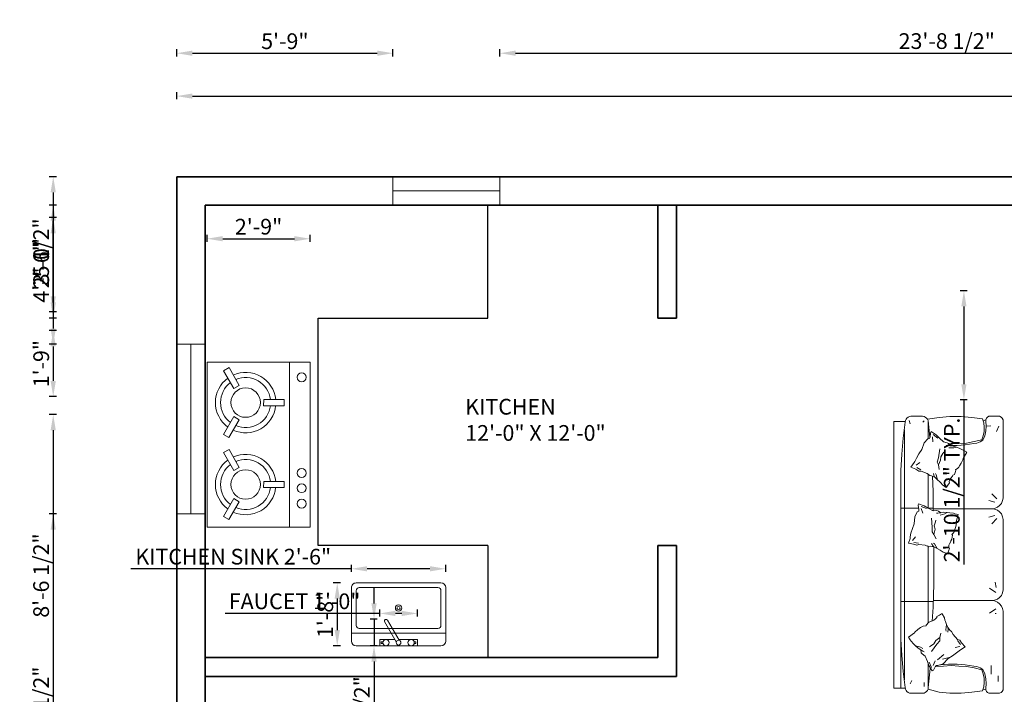
# Model space of a CAD drawing. Units: inches. Extents: x -48 to 817, y -530 to 78.
# Tile 3 of 7: x -48 to 266, y -153 to 62. Entities that reach past the tile are written whole.
import ezdxf

# ---------------------------------------------------------------- set-up
doc = ezdxf.new("R2010")
doc.units = ezdxf.units.IN
for name, color, linetype, lineweight in [('A-ANNO-DIMS', 2, 'Continuous', 18), ('A-AREA-IDEN', 7, 'Continuous', 18), ('A-EQPM', 8, 'Continuous', 18), ('A-FLOR-CASE', 8, 'Continuous', 25), ('A-FLOR-FIXT', 9, 'Continuous', 18), ('A-GLAZ', 4, 'Continuous', 18), ('A-WALL', 7, 'Continuous', 35), ('furn', 8, 'Continuous', 18)]:
    doc.layers.add(name, color=color, linetype=linetype, lineweight=lineweight)
doc.styles.get("Standard").update_dxf_attribs({"font": 'arial.ttf'})
doc.dimstyles.new('ISO-25', dxfattribs={"dimtxt": 5, "dimasz": 5, "dimexe": 1.25, "dimexo": 0.625, "dimtad": 1, "dimlunit": 3, "dimtxsty": 'Standard', "dimcen": 2.5, "dimadec": 0, "dimazin": 0, "dimtfac": 1, "dimtmove": 0, "dimatfit": 3, "dimfxl": 1, "dimfxlon": 1, "dimarcsym": 0})

# ---------------------------------------------------------------- blocks, each defined once
blk = doc.blocks.new('Sink-single - 30 in top')
blk.add_line((-15, -3.999996), (15, -3.999996))
for points in [[(-13.5, 0), (13.5, 0)], [(-15, -18.499996), (-15, -1.5)], [(15, -1.5), (15, -18.499996)], [(-12.5, -5.499996), (12.5, -5.499996)], [(-13.5, -17.499996), (-13.5, -6.499996)], [(13.5, -6.499996), (13.5, -17.499996)], [(12.5, -18.499996), (-12.5, -18.499996)], [(13.5, -19.999996), (-13.5, -19.999996)]]:
    blk.add_lwpolyline(points)
for radius in [1, 0.5]:
    blk.add_circle((0, -11.999996), radius)
for centre, radius, start, end in [((-13.5, -1.5), 1.5, 90, 180), ((13.5, -1.5), 1.5, 0, 90), ((-12.5, -6.499996), 1, 90, 180), ((12.5, -6.499996), 1, 0, 90), ((-13.5, -18.499996), 1.5, 180, 270), ((-12.5, -17.499996), 1, 180, 270), ((12.5, -17.499996), 1, 270, 0), ((13.5, -18.499996), 1.5, 270, 0)]:
    blk.add_arc(centre, radius, start, end)
blk = doc.blocks.new('Faucet - kit sink top')
for p, q in [((-5.5, -0.75), (-5.5, -1.25)), ((-4.94278, -0.75), (-5.5, -0.75)), ((-5.5, -1.25), (-4.94278, -1.25)), ((-0.14775, -1.7441), (3.56698, -8.1782)), ((4.43301, -7.6782), (0.71828, -1.2441)), ((4.94278, -0.75), (5.5, -0.75)), ((5.5, -1.25), (4.94278, -1.25)), ((5.5, -0.75), (5.5, -1.25))]:
    blk.add_line(p, q)
blk.add_lwpolyline([(-0.00587, -2), (-6, -2), (-6, 0), (6, 0), (6, -2), (1.15195, -2)])
for centre, radius in [((-4, -1), 1), ((4, -1), 1), ((0, -1), 0.75)]:
    blk.add_circle(centre, radius)
blk.add_arc((4, -7.9282), 0.5, 210, 30)
blk = doc.blocks.new('sofa-43')
at = {"color": 0, "linetype": 'ByBlock'}
for p, q in [((-0.015, 0.947), (-0.028, 0.939)), ((-0.028, 0.939), (-0.015, 0.947)), ((-0.003, 0.947), (-0.015, 0.947)), ((-0.015, 0.947), (-0.003, 0.947)), ((0.665, 0.947), (-0.003, 0.947)), ((-0.003, 0.947), (0.665, 0.947)), ((0.687, 0.942), (0.665, 0.947)), ((0.687, 0.942), (0.665, 0.947)), ((0.712, 0.932), (0.687, 0.942)), ((0.712, 0.932), (0.687, 0.942)), ((0.827, 0.942), (0.802, 0.932)), ((0.802, 0.932), (0.827, 0.942)), ((0.85, 0.947), (0.827, 0.942)), ((0.827, 0.942), (0.85, 0.947)), ((1.462, 0.947), (0.85, 0.947)), ((0.85, 0.947), (1.462, 0.947)), ((1.487, 0.942), (1.462, 0.947)), ((1.487, 0.942), (1.462, 0.947)), ((1.509, 0.932), (1.487, 0.942)), ((1.509, 0.932), (1.487, 0.942)), ((1.624, 0.942), (1.602, 0.932)), ((1.602, 0.932), (1.624, 0.942)), ((1.647, 0.947), (1.624, 0.942)), ((1.624, 0.942), (1.647, 0.947)), ((2.317, 0.947), (1.647, 0.947)), ((1.647, 0.947), (2.317, 0.947)), ((2.329, 0.947), (2.317, 0.947)), ((2.329, 0.947), (2.317, 0.947)), ((2.342, 0.939), (2.329, 0.947)), ((2.342, 0.939), (2.329, 0.947)), ((-0.038, 0.929), (-0.045, 0.917)), ((-0.045, 0.917), (-0.038, 0.929)), ((-0.045, 0.917), (-0.045, 0.824)), ((-0.045, 0.917), (-0.045, 0.824)), ((-0.028, 0.939), (-0.038, 0.929)), ((-0.038, 0.929), (-0.028, 0.939)), ((0.042, 0.909), (0.087, 0.889)), ((0.672, 0.892), (0.627, 0.849)), ((0.7, 0.874), (0.685, 0.824)), ((0.73, 0.917), (0.712, 0.932)), ((0.73, 0.917), (0.712, 0.932)), ((0.745, 0.897), (0.73, 0.917)), ((0.745, 0.897), (0.73, 0.917)), ((0.755, 0.872), (0.745, 0.897)), ((0.755, 0.872), (0.745, 0.897)), ((0.757, 0.849), (0.755, 0.872)), ((0.757, 0.849), (0.755, 0.872)), ((0.76, 0.872), (0.757, 0.849)), ((0.757, 0.849), (0.76, 0.872)), ((0.77, 0.897), (0.76, 0.872)), ((0.76, 0.872), (0.77, 0.897)), ((0.785, 0.917), (0.77, 0.897)), ((0.77, 0.897), (0.785, 0.917)), ((0.802, 0.932), (0.785, 0.917)), ((0.785, 0.917), (0.802, 0.932)), ((0.815, 0.874), (0.83, 0.824)), ((0.842, 0.892), (0.887, 0.849)), ((1.442, 0.887), (1.394, 0.877)), ((1.484, 0.884), (1.447, 0.829)), ((1.527, 0.917), (1.509, 0.932)), ((1.527, 0.917), (1.509, 0.932)), ((1.542, 0.897), (1.527, 0.917)), ((1.542, 0.897), (1.527, 0.917)), ((1.552, 0.872), (1.542, 0.897)), ((1.552, 0.872), (1.542, 0.897)), ((1.554, 0.849), (1.552, 0.872)), ((1.554, 0.849), (1.552, 0.872)), ((1.557, 0.872), (1.554, 0.849)), ((1.554, 0.849), (1.557, 0.872)), ((1.567, 0.897), (1.557, 0.872)), ((1.557, 0.872), (1.567, 0.897)), ((1.582, 0.917), (1.567, 0.897)), ((1.567, 0.897), (1.582, 0.917)), ((1.602, 0.932), (1.582, 0.917)), ((1.582, 0.917), (1.602, 0.932)), ((1.627, 0.884), (1.664, 0.829)), ((1.667, 0.887), (1.667, 0.877)), ((2.257, 0.904), (2.207, 0.904)), ((2.352, 0.929), (2.342, 0.939)), ((2.352, 0.929), (2.342, 0.939)), ((2.359, 0.917), (2.352, 0.929)), ((2.359, 0.917), (2.352, 0.929)), ((2.359, 0.824), (2.359, 0.917)), ((2.359, 0.917), (2.359, 0.824)), ((-0.045, 0.824), (-0.038, 0.812)), ((-0.045, 0.824), (-0.038, 0.812)), ((-0.038, 0.812), (-0.028, 0.802)), ((-0.038, 0.812), (-0.028, 0.802)), ((-0.023, 0.769), (-0.035, 0.677)), ((-0.023, 0.769), (-0.035, 0.677)), ((-0.028, 0.802), (-0.015, 0.797)), ((-0.028, 0.802), (-0.015, 0.797)), ((0.012, 0.779), (-0.023, 0.769)), ((-0.0064, 0.7737), (-0.023, 0.769)), ((-0.015, 0.797), (-0.0064, 0.7737)), ((-0.015, 0.797), (-0.003, 0.797)), ((-0.0064, 0.7737), (-0.015, 0.797)), ((0.04, 0.799), (-0.003, 0.797)), ((0.05, 0.782), (0.012, 0.779)), ((0.04, 0.799), (0.037, 0.839)), ((0.082, 0.797), (0.04, 0.799)), ((0.087, 0.782), (0.05, 0.782)), ((0.125, 0.787), (0.082, 0.797)), ((0.125, 0.774), (0.087, 0.782)), ((0.162, 0.772), (0.125, 0.787)), ((0.16, 0.762), (0.125, 0.774)), ((0.177, 0.747), (0.162, 0.772)), ((0.757, 0.345), (0.757, 0.849)), ((1.554, 0.345), (1.554, 0.849)), ((2.194, 0.842), (2.119, 0.842)), ((2.137, 0.747), (2.152, 0.772)), ((2.152, 0.772), (2.189, 0.787)), ((2.154, 0.762), (2.189, 0.774)), ((2.189, 0.787), (2.232, 0.797)), ((2.189, 0.774), (2.227, 0.782)), ((2.227, 0.782), (2.264, 0.782)), ((2.232, 0.797), (2.274, 0.799)), ((2.264, 0.782), (2.302, 0.779)), ((2.274, 0.799), (2.317, 0.797)), ((2.302, 0.779), (2.337, 0.769)), ((2.329, 0.797), (2.317, 0.797)), ((2.3218, 0.7734), (2.329, 0.797)), ((2.3218, 0.7734), (2.329, 0.797)), ((2.337, 0.769), (2.3218, 0.7734)), ((2.329, 0.797), (2.342, 0.802)), ((2.342, 0.802), (2.329, 0.797)), ((2.349, 0.677), (2.337, 0.769)), ((2.337, 0.769), (2.349, 0.677)), ((2.342, 0.802), (2.352, 0.812)), ((2.352, 0.812), (2.342, 0.802)), ((2.352, 0.812), (2.359, 0.824)), ((2.359, 0.824), (2.352, 0.812)), ((0.175, 0.697), (0.16, 0.762)), ((0.187, 0.629), (0.175, 0.697)), ((0.187, 0.719), (0.177, 0.747)), ((0.192, 0.692), (0.187, 0.719)), ((0.202, 0.619), (0.192, 0.692)), ((2.112, 0.619), (2.122, 0.692)), ((2.122, 0.692), (2.127, 0.719)), ((2.127, 0.719), (2.137, 0.747)), ((2.127, 0.629), (2.139, 0.697)), ((2.139, 0.697), (2.154, 0.762)), ((-0.035, 0.677), (-0.043, 0.582)), ((-0.035, 0.677), (-0.043, 0.582)), ((0.192, 0.562), (0.187, 0.629)), ((0.207, 0.547), (0.202, 0.619)), ((0.252, 0.607), (0.245, 0.594)), ((0.267, 0.632), (0.252, 0.607)), ((0.322, 0.599), (0.267, 0.632)), ((0.332, 0.597), (0.322, 0.599)), ((1.957, 0.617), (1.922, 0.587)), ((1.982, 0.577), (1.957, 0.617)), ((2.107, 0.547), (2.112, 0.619)), ((2.122, 0.562), (2.127, 0.629)), ((2.357, 0.582), (2.349, 0.677)), ((2.349, 0.677), (2.357, 0.582)), ((-0.043, 0.582), (-0.043, 0.484)), ((-0.043, 0.582), (-0.043, 0.484)), ((0.195, 0.497), (0.192, 0.562)), ((0.207, 0.492), (0.207, 0.547)), ((0.215, 0.514), (0.212, 0.487)), ((0.222, 0.542), (0.215, 0.514)), ((0.232, 0.567), (0.222, 0.542)), ((0.222, 0.542), (0.23, 0.519)), ((0.23, 0.519), (0.23, 0.497)), ((0.245, 0.594), (0.232, 0.567)), ((0.362, 0.584), (0.332, 0.597)), ((0.385, 0.569), (0.362, 0.584)), ((0.397, 0.562), (0.385, 0.569)), ((0.405, 0.554), (0.397, 0.562)), ((0.42, 0.534), (0.405, 0.554)), ((0.425, 0.537), (0.42, 0.534)), ((0.46, 0.524), (0.425, 0.537)), ((0.467, 0.512), (0.46, 0.524)), ((0.797, 0.517), (0.792, 0.484)), ((0.8, 0.529), (0.797, 0.517)), ((0.807, 0.557), (0.8, 0.529)), ((0.87, 0.539), (0.807, 0.557)), ((0.88, 0.542), (0.87, 0.539)), ((0.912, 0.537), (0.88, 0.542)), ((0.937, 0.529), (0.912, 0.537)), ((0.952, 0.524), (0.937, 0.529)), ((0.962, 0.519), (0.952, 0.524)), ((0.982, 0.502), (0.962, 0.519)), ((1.849, 0.514), (1.822, 0.499)), ((1.892, 0.552), (1.849, 0.514)), ((1.899, 0.572), (1.892, 0.552)), ((1.922, 0.587), (1.899, 0.572)), ((1.934, 0.577), (1.902, 0.552)), ((1.954, 0.572), (1.962, 0.532)), ((1.989, 0.567), (1.982, 0.577)), ((2.009, 0.542), (1.989, 0.567)), ((2.034, 0.507), (2.009, 0.542)), ((2.107, 0.474), (2.107, 0.547)), ((2.119, 0.497), (2.122, 0.562)), ((2.357, 0.484), (2.357, 0.582)), ((2.357, 0.582), (2.357, 0.484)), ((-0.043, 0.484), (-0.035, 0.392)), ((-0.043, 0.484), (-0.035, 0.392)), ((0.177, 0.43), (0.145, 0.395)), ((0.185, 0.462), (0.177, 0.43)), ((0.192, 0.472), (0.185, 0.462)), ((0.212, 0.487), (0.192, 0.472)), ((0.195, 0.482), (0.195, 0.497)), ((0.207, 0.467), (0.212, 0.487)), ((0.207, 0.452), (0.207, 0.467)), ((0.23, 0.497), (0.23, 0.477)), ((0.277, 0.425), (0.265, 0.432)), ((0.475, 0.507), (0.467, 0.512)), ((0.492, 0.492), (0.475, 0.507)), ((0.507, 0.484), (0.492, 0.492)), ((0.522, 0.479), (0.507, 0.484)), ((0.532, 0.482), (0.522, 0.479)), ((0.552, 0.467), (0.532, 0.482)), ((0.55, 0.422), (0.572, 0.452)), ((0.57, 0.457), (0.552, 0.467)), ((0.572, 0.452), (0.57, 0.457)), ((0.79, 0.462), (0.787, 0.432)), ((0.787, 0.432), (0.792, 0.407)), ((0.792, 0.484), (0.79, 0.462)), ((0.79, 0.462), (0.802, 0.442)), ((0.802, 0.442), (0.807, 0.42)), ((0.987, 0.507), (0.982, 0.502)), ((1.022, 0.502), (0.987, 0.507)), ((1.035, 0.492), (1.022, 0.502)), ((1.042, 0.492), (1.035, 0.492)), ((1.062, 0.482), (1.042, 0.492)), ((1.074, 0.477), (1.062, 0.482)), ((1.092, 0.477), (1.074, 0.477)), ((1.102, 0.482), (1.092, 0.477)), ((1.124, 0.472), (1.102, 0.482)), ((1.144, 0.467), (1.124, 0.472)), ((1.134, 0.427), (1.147, 0.465)), ((1.147, 0.465), (1.144, 0.467)), ((1.704, 0.437), (1.669, 0.417)), ((1.724, 0.442), (1.704, 0.437)), ((1.737, 0.447), (1.724, 0.442)), ((1.762, 0.457), (1.737, 0.447)), ((1.789, 0.467), (1.762, 0.457)), ((1.762, 0.457), (1.807, 0.45)), ((1.814, 0.487), (1.789, 0.467)), ((1.789, 0.467), (1.802, 0.47)), ((1.802, 0.47), (1.827, 0.467)), ((1.807, 0.45), (1.819, 0.452)), ((1.822, 0.499), (1.814, 0.487)), ((1.827, 0.504), (1.832, 0.502)), ((2.069, 0.377), (2.022, 0.432)), ((2.057, 0.47), (2.034, 0.507)), ((2.062, 0.422), (2.049, 0.479)), ((2.102, 0.427), (2.057, 0.47)), ((2.112, 0.405), (2.107, 0.474)), ((2.122, 0.43), (2.119, 0.497)), ((2.127, 0.362), (2.122, 0.43)), ((2.349, 0.392), (2.357, 0.484)), ((2.357, 0.484), (2.349, 0.392)), ((-0.035, 0.392), (-0.02, 0.292)), ((-0.035, 0.392), (-0.02, 0.292)), ((0.117, 0.367), (0.087, 0.322)), ((0.112, 0.34), (0.145, 0.38)), ((0.145, 0.395), (0.117, 0.367)), ((0.237, 0.397), (0.315, 0.385)), ((0.307, 0.407), (0.277, 0.425)), ((0.337, 0.405), (0.307, 0.407)), ((0.315, 0.385), (0.352, 0.375)), ((0.377, 0.387), (0.337, 0.405)), ((0.352, 0.375), (0.377, 0.387)), ((0.377, 0.387), (0.417, 0.392)), ((0.462, 0.367), (0.452, 0.36)), ((0.477, 0.35), (0.452, 0.342)), ((0.505, 0.377), (0.462, 0.367)), ((0.472, 0.327), (0.485, 0.357)), ((0.485, 0.357), (0.477, 0.35)), ((0.485, 0.357), (0.505, 0.377)), ((0.505, 0.377), (0.525, 0.397)), ((0.525, 0.397), (0.532, 0.407)), ((0.532, 0.407), (0.55, 0.422)), ((0.777, 0.385), (0.772, 0.372)), ((0.772, 0.372), (0.775, 0.34)), ((0.792, 0.407), (0.777, 0.385)), ((0.795, 0.382), (0.792, 0.407)), ((0.797, 0.37), (0.795, 0.382)), ((0.807, 0.42), (0.812, 0.4)), ((0.872, 0.36), (0.857, 0.362)), ((0.905, 0.35), (0.872, 0.36)), ((0.935, 0.357), (0.905, 0.35)), ((0.98, 0.347), (0.935, 0.357)), ((0.957, 0.33), (0.98, 0.347)), ((0.98, 0.347), (1.017, 0.365)), ((1.062, 0.352), (1.057, 0.342)), ((1.102, 0.375), (1.062, 0.352)), ((1.087, 0.347), (1.082, 0.34)), ((1.082, 0.317), (1.087, 0.347)), ((1.087, 0.347), (1.102, 0.375)), ((1.409, 0.347), (1.087, 0.347)), ((1.102, 0.375), (1.117, 0.4)), ((1.117, 0.4), (1.122, 0.41)), ((1.122, 0.41), (1.134, 0.427)), ((1.612, 0.34), (1.409, 0.347)), ((1.669, 0.417), (1.669, 0.412)), ((1.669, 0.412), (1.682, 0.395)), ((1.682, 0.395), (1.692, 0.372)), ((1.692, 0.372), (1.702, 0.372)), ((1.702, 0.372), (1.714, 0.36)), ((1.714, 0.36), (1.724, 0.347)), ((1.724, 0.347), (1.734, 0.325)), ((1.874, 0.397), (1.837, 0.407)), ((1.874, 0.397), (1.902, 0.362)), ((1.904, 0.397), (1.874, 0.397)), ((1.902, 0.362), (1.929, 0.347)), ((1.932, 0.372), (1.904, 0.397)), ((1.929, 0.347), (1.949, 0.317)), ((1.997, 0.325), (1.932, 0.372)), ((2.119, 0.34), (2.077, 0.357)), ((2.119, 0.382), (2.102, 0.427)), ((2.117, 0.375), (2.112, 0.405)), ((2.117, 0.37), (2.119, 0.382)), ((2.124, 0.36), (2.117, 0.37)), ((2.157, 0.342), (2.124, 0.36)), ((2.129, 0.357), (2.127, 0.362)), ((2.164, 0.332), (2.157, 0.342)), ((2.322, 0.297), (2.349, 0.392)), ((2.349, 0.392), (2.322, 0.297)), ((-0.043, 0.262), (-0.045, 0.247)), ((-0.043, 0.262), (-0.045, 0.247)), ((-0.038, 0.272), (-0.043, 0.262)), ((-0.038, 0.272), (-0.043, 0.262)), ((-0.03, 0.282), (-0.038, 0.272)), ((-0.03, 0.282), (-0.038, 0.272)), ((-0.02, 0.292), (-0.03, 0.282)), ((-0.02, 0.292), (-0.03, 0.282)), ((-0.008, 0.297), (-0.02, 0.292)), ((0.14, 0.312), (-0.008, 0.297)), ((-0.008, 0.297), (0.15, 0.297)), ((0.005, 0.297), (-0.008, 0.297)), ((-0.005, 0.262), (0.007, 0.25)), ((0.087, 0.322), (0.1, 0.317)), ((0.1, 0.317), (0.135, 0.315)), ((0.132, 0.335), (0.177, 0.337)), ((0.135, 0.315), (0.147, 0.307)), ((0.147, 0.307), (0.152, 0.295)), ((0.152, 0.295), (0.185, 0.262)), ((0.185, 0.262), (0.242, 0.242)), ((0.43, 0.235), (0.452, 0.287)), ((0.452, 0.287), (0.47, 0.312)), ((0.46, 0.297), (0.752, 0.297)), ((0.467, 0.307), (0.462, 0.307)), ((0.47, 0.312), (0.472, 0.327)), ((0.607, 0.34), (0.475, 0.335)), ((0.775, 0.34), (0.607, 0.34)), ((0.732, 0.262), (0.715, 0.212)), ((0.752, 0.297), (0.732, 0.262)), ((0.737, 0.237), (0.755, 0.282)), ((0.775, 0.34), (0.752, 0.297)), ((0.752, 0.297), (0.752, 0.34)), ((0.84, 0.325), (0.917, 0.33)), ((0.917, 0.33), (0.957, 0.33)), ((1.082, 0.34), (1.059, 0.327)), ((1.067, 0.217), (1.074, 0.272)), ((1.074, 0.272), (1.087, 0.302)), ((1.084, 0.297), (1.079, 0.292)), ((1.087, 0.302), (1.082, 0.317)), ((1.0855, 0.2985), (1.084, 0.297)), ((1.084, 0.297), (1.0848, 0.297)), ((1.084, 0.297), (1.562, 0.297)), ((1.0848, 0.297), (1.0855, 0.2985)), ((1.562, 0.06), (1.562, 0.34)), ((1.562, 0.297), (1.747, 0.297)), ((1.732, 0.332), (1.612, 0.34)), ((1.734, 0.325), (1.737, 0.32)), ((1.737, 0.32), (1.742, 0.302)), ((1.742, 0.302), (1.767, 0.28)), ((1.767, 0.28), (1.772, 0.28)), ((1.772, 0.28), (1.777, 0.252)), ((1.949, 0.317), (1.957, 0.307)), ((1.999, 0.262), (1.994, 0.25)), ((2.017, 0.245), (2.037, 0.272)), ((2.037, 0.272), (2.082, 0.29)), ((2.082, 0.29), (2.119, 0.302)), ((2.134, 0.327), (2.089, 0.305)), ((2.104, 0.297), (2.309, 0.297)), ((2.117, 0.317), (2.114, 0.317)), ((2.119, 0.302), (2.164, 0.332)), ((2.144, 0.315), (2.137, 0.317)), ((2.137, 0.315), (2.137, 0.317)), ((2.309, 0.297), (2.144, 0.315)), ((2.299, 0.262), (2.264, 0.262)), ((2.322, 0.297), (2.309, 0.297)), ((2.334, 0.292), (2.322, 0.297)), ((2.334, 0.292), (2.322, 0.297)), ((2.344, 0.282), (2.334, 0.292)), ((2.344, 0.282), (2.334, 0.292)), ((2.352, 0.272), (2.344, 0.282)), ((2.352, 0.272), (2.344, 0.282)), ((2.357, 0.262), (2.352, 0.272)), ((2.357, 0.262), (2.352, 0.272)), ((2.359, 0.247), (2.357, 0.262)), ((2.359, 0.247), (2.357, 0.262)), ((-0.045, 0.247), (-0.045, 0.147)), ((-0.045, 0.247), (-0.045, 0.147)), ((0.242, 0.242), (0.28, 0.215)), ((0.28, 0.215), (0.317, 0.195)), ((0.317, 0.195), (0.347, 0.182)), ((0.347, 0.182), (0.357, 0.175)), ((0.38, 0.192), (0.355, 0.225)), ((0.357, 0.175), (0.397, 0.147)), ((0.397, 0.147), (0.415, 0.19)), ((0.4, 0.197), (0.42, 0.232)), ((0.415, 0.19), (0.43, 0.215)), ((0.43, 0.215), (0.43, 0.235)), ((0.715, 0.212), (0.727, 0.21)), ((0.727, 0.21), (0.765, 0.217)), ((0.752, 0.06), (0.752, 0.215)), ((0.755, 0.237), (0.797, 0.25)), ((0.765, 0.217), (0.777, 0.215)), ((0.777, 0.215), (0.785, 0.202)), ((0.785, 0.202), (0.827, 0.18)), ((0.827, 0.18), (0.887, 0.175)), ((0.887, 0.175), (0.93, 0.16)), ((1.032, 0.162), (1, 0.187)), ((1.05, 0.172), (1.057, 0.212)), ((1.064, 0.17), (1.072, 0.197)), ((1.072, 0.197), (1.067, 0.217)), ((1.777, 0.252), (1.782, 0.242)), ((1.782, 0.242), (1.789, 0.23)), ((1.789, 0.23), (1.804, 0.207)), ((1.804, 0.207), (1.827, 0.182)), ((1.827, 0.182), (1.834, 0.177)), ((1.834, 0.177), (1.872, 0.125)), ((1.929, 0.17), (1.947, 0.187)), ((1.947, 0.187), (1.952, 0.212)), ((1.947, 0.187), (1.967, 0.21)), ((1.952, 0.212), (1.959, 0.23)), ((1.959, 0.23), (1.969, 0.25)), ((1.967, 0.21), (1.982, 0.232)), ((1.994, 0.25), (1.982, 0.232)), ((1.982, 0.232), (2.007, 0.237)), ((2.007, 0.237), (2.017, 0.245)), ((2.359, 0.147), (2.359, 0.247)), ((2.359, 0.147), (2.359, 0.247)), ((-0.045, 0.147), (-0.043, 0.135)), ((-0.045, 0.147), (-0.043, 0.135)), ((-0.043, 0.135), (-0.038, 0.122)), ((-0.043, 0.135), (-0.038, 0.122)), ((-0.038, 0.122), (-0.03, 0.112)), ((-0.038, 0.122), (-0.03, 0.112)), ((-0.03, 0.112), (-0.02, 0.105)), ((-0.03, 0.112), (-0.02, 0.105)), ((-0.02, 0.105), (-0.008, 0.1)), ((-0.02, 0.105), (-0.008, 0.1)), ((-0.008, 0.132), (0.02, 0.142)), ((-0.008, 0.1), (0, 0.0982)), ((-0.008, 0.1), (0.005, 0.097)), ((0, 0.1), (0, 0)), ((0, 0.0982), (0, 0)), ((0.005, 0.097), (0.145, 0.08)), ((0.072, 0.09), (0.752, 0.09)), ((0.752, 0.09), (1.562, 0.09)), ((0.93, 0.16), (0.97, 0.147)), ((0.97, 0.147), (1.002, 0.142)), ((1.002, 0.142), (1.015, 0.14)), ((1.015, 0.14), (1.057, 0.125)), ((1.057, 0.125), (1.064, 0.17)), ((1.562, 0.09), (2.242, 0.09)), ((1.872, 0.125), (1.894, 0.142)), ((1.894, 0.142), (1.907, 0.15)), ((1.907, 0.15), (1.929, 0.17)), ((2.169, 0.08), (2.309, 0.097)), ((2.277, 0.142), (2.249, 0.155)), ((2.309, 0.097), (2.322, 0.1)), ((2.314, 0.0982), (2.322, 0.1)), ((2.314, 0.1), (2.314, 0)), ((2.314, 0), (2.314, 0.0982)), ((2.322, 0.1), (2.334, 0.105)), ((2.322, 0.1), (2.334, 0.105)), ((2.334, 0.105), (2.344, 0.112)), ((2.334, 0.105), (2.344, 0.112)), ((2.344, 0.112), (2.352, 0.122)), ((2.344, 0.112), (2.352, 0.122)), ((2.352, 0.122), (2.357, 0.135)), ((2.352, 0.122), (2.357, 0.135)), ((2.357, 0.135), (2.359, 0.147)), ((2.357, 0.135), (2.359, 0.147)), ((0, 0), (2.314, 0)), ((0, 0), (2.314, 0)), ((0.145, 0.08), (0.285, 0.067)), ((0.285, 0.067), (0.425, 0.06)), ((0.425, 0.06), (2.314, 0.06)), ((1.889, 0.06), (2.029, 0.067)), ((2.029, 0.067), (2.169, 0.08))]:
    blk.add_line(p, q, dxfattribs=at)
blk = doc.blocks.new('*D9')
at = {"layer": 'A-ANNO-DIMS', "color": 0, "lineweight": -2, "transparency": 16777216}
for p, q in [((2.43, 36.38), (2.43, 38.63)), ((722.43, 36.38), (722.43, 38.63)), ((7.43, 37.38), (717.43, 37.38))]:
    blk.add_line(p, q, dxfattribs=at)
at = {"layer": 'A-ANNO-DIMS', "color": 0, "transparency": 16777216}
for points in [[(7.43, 38.21), (7.43, 36.54), (2.43, 37.38)], [(717.43, 38.21), (717.43, 36.54), (722.43, 37.38)]]:
    blk.add_solid(points, dxfattribs=at)
at = {"layer": 'Defpoints', "color": 0, "transparency": 16777216}
for p in [(722.43, 37.38), (2.43, 11.72), (722.43, 11.72)]:
    blk.add_point(p, dxfattribs=at)
at = {"layer": 'A-ANNO-DIMS', "color": 0, "transparency": 16777216, "insert": (362.43, 40.55), "char_height": 5, "attachment_point": 5}
blk.add_mtext("60'", dxfattribs=at)
blk = doc.blocks.new('WIN-54IN')
blk.add_line((4.5, 54), (4.5, 0))
blk.add_lwpolyline([(9, 54), (0, 54), (0, 0), (9, 0)], close=True)
blk = doc.blocks.new('WIN-34IN')
blk.add_line((4.5, 34), (4.5, 0))
blk.add_lwpolyline([(9, 34), (0, 34), (0, 0), (9, 0)], close=True)
blk = doc.blocks.new('*D27')
at = {"layer": 'A-ANNO-DIMS', "color": 0, "lineweight": -2, "transparency": 16777216}
for p, q in [((253.82, -24.56), (251.57, -24.56)), ((252.82, -29.56), (252.82, -54.28)), ((253.82, -59.28), (251.57, -59.28)), ((252.82, -59.28), (252.82, -111.62))]:
    blk.add_line(p, q, dxfattribs=at)
at = {"layer": 'A-ANNO-DIMS', "color": 0, "transparency": 16777216}
for points in [[(251.99, -29.56), (253.65, -29.56), (252.82, -24.56)], [(251.99, -54.28), (253.65, -54.28), (252.82, -59.28)]]:
    blk.add_solid(points, dxfattribs=at)
at = {"layer": 'Defpoints', "color": 0, "transparency": 16777216}
for p in [(266.04, -24.56), (252.82, -59.28), (266.04, -59.28)]:
    blk.add_point(p, dxfattribs=at)
at = {"layer": 'A-ANNO-DIMS', "color": 0, "transparency": 16777216, "insert": (249.61, -87.95), "char_height": 5, "attachment_point": 5, "rotation": 90}
blk.add_mtext('2\'-10 1/2" TYP.', dxfattribs=at)
blk = doc.blocks.new('*D38')
at = {"layer": 'A-ANNO-DIMS', "color": 0, "lineweight": -2, "transparency": 16777216}
for p, q in [((57.97, -114.02), (57.97, -111.77)), ((87.97, -114.02), (87.97, -111.77)), ((57.97, -113.02), (-12.19, -113.02)), ((82.97, -113.02), (62.97, -113.02))]:
    blk.add_line(p, q, dxfattribs=at)
at = {"layer": 'A-ANNO-DIMS', "color": 0, "transparency": 16777216}
for points in [[(62.97, -112.19), (62.97, -113.85), (57.97, -113.02)], [(82.97, -112.19), (82.97, -113.85), (87.97, -113.02)]]:
    blk.add_solid(points, dxfattribs=at)
at = {"layer": 'Defpoints', "color": 0, "transparency": 16777216}
for p in [(57.97, -113.02), (57.97, -117.52), (87.97, -117.52)]:
    blk.add_point(p, dxfattribs=at)
at = {"layer": 'A-ANNO-DIMS', "color": 0, "transparency": 16777216, "insert": (20.39, -109.81), "char_height": 5, "attachment_point": 5}
blk.add_mtext('KITCHEN SINK 2\'-6"', dxfattribs=at)
blk = doc.blocks.new('*D39')
at = {"layer": 'A-ANNO-DIMS', "color": 0, "lineweight": -2, "transparency": 16777216}
for p, q in [((54.47, -117.52), (52.22, -117.52)), ((53.47, -122.52), (53.47, -132.52)), ((54.47, -137.52), (52.22, -137.52))]:
    blk.add_line(p, q, dxfattribs=at)
at = {"layer": 'A-ANNO-DIMS', "color": 0, "transparency": 16777216}
for points in [[(52.64, -122.52), (54.31, -122.52), (53.47, -117.52)], [(52.64, -132.52), (54.31, -132.52), (53.47, -137.52)]]:
    blk.add_solid(points, dxfattribs=at)
at = {"layer": 'Defpoints', "color": 0, "transparency": 16777216}
for p in [(57.97, -117.52), (53.47, -137.52), (57.97, -137.52)]:
    blk.add_point(p, dxfattribs=at)
at = {"layer": 'A-ANNO-DIMS', "color": 0, "transparency": 16777216, "insert": (50.3, -127.52), "char_height": 5, "attachment_point": 5, "rotation": 90}
blk.add_mtext('1\'-8"', dxfattribs=at)
blk = doc.blocks.new('*D40')
at = {"layer": 'A-ANNO-DIMS', "color": 0, "lineweight": -2, "transparency": 16777216}
for p, q in [((66.97, -127.22), (17.84, -127.22)), ((66.97, -128.22), (66.97, -125.97)), ((73.97, -127.22), (71.97, -127.22)), ((78.97, -128.22), (78.97, -125.97))]:
    blk.add_line(p, q, dxfattribs=at)
at = {"layer": 'A-ANNO-DIMS', "color": 0, "transparency": 16777216}
for points in [[(71.97, -126.39), (71.97, -128.05), (66.97, -127.22)], [(73.97, -126.39), (73.97, -128.05), (78.97, -127.22)]]:
    blk.add_solid(points, dxfattribs=at)
at = {"layer": 'Defpoints', "color": 0, "transparency": 16777216}
for p in [(66.97, -127.22), (66.97, -129.02), (78.97, -129.02)]:
    blk.add_point(p, dxfattribs=at)
at = {"layer": 'A-ANNO-DIMS', "color": 0, "transparency": 16777216, "insert": (39.91, -124.01), "char_height": 5, "attachment_point": 5}
blk.add_mtext('FAUCET 1\'-0"', dxfattribs=at)
blk = doc.blocks.new('*D41')
at = {"layer": 'A-ANNO-DIMS', "color": 0, "lineweight": -2, "transparency": 16777216}
for p, q in [((65.17, -124.02), (65.17, -119.02)), ((66.17, -129.02), (63.92, -129.02)), ((65.17, -129.02), (65.17, -137.52)), ((66.17, -137.52), (63.92, -137.52)), ((65.17, -142.52), (65.17, -173.71))]:
    blk.add_line(p, q, dxfattribs=at)
at = {"layer": 'A-ANNO-DIMS', "color": 0, "transparency": 16777216}
for points in [[(64.34, -124.02), (66.01, -124.02), (65.17, -129.02)], [(64.34, -142.52), (66.01, -142.52), (65.17, -137.52)]]:
    blk.add_solid(points, dxfattribs=at)
at = {"layer": 'Defpoints', "color": 0, "transparency": 16777216}
for p in [(66.97, -129.02), (65.17, -137.52), (66.97, -137.52)]:
    blk.add_point(p, dxfattribs=at)
at = {"layer": 'A-ANNO-DIMS', "color": 0, "transparency": 16777216, "insert": (61.96, -160.61), "char_height": 5, "attachment_point": 5, "rotation": 90}
blk.add_mtext('0\'-8 1/2"', dxfattribs=at)
blk = doc.blocks.new('*D47')
at = {"layer": 'A-ANNO-DIMS', "color": 0, "lineweight": -2, "transparency": 16777216}
for p, q in [((2.43, 50.02), (2.43, 52.27)), ((7.43, 51.02), (66.2, 51.02)), ((71.2, 50.02), (71.2, 52.27))]:
    blk.add_line(p, q, dxfattribs=at)
at = {"layer": 'A-ANNO-DIMS', "color": 0, "transparency": 16777216}
for points in [[(7.43, 51.86), (7.43, 50.19), (2.43, 51.02)], [(66.2, 51.86), (66.2, 50.19), (71.2, 51.02)]]:
    blk.add_solid(points, dxfattribs=at)
at = {"layer": 'Defpoints', "color": 0, "transparency": 16777216}
for p in [(71.2, 51.02), (2.43, 11.72), (71.2, 11.72)]:
    blk.add_point(p, dxfattribs=at)
at = {"layer": 'A-ANNO-DIMS', "color": 0, "transparency": 16777216, "insert": (36.81, 54.2), "char_height": 5, "attachment_point": 5}
blk.add_mtext('5\'-9"', dxfattribs=at)
blk = doc.blocks.new('*D48')
at = {"layer": 'A-ANNO-DIMS', "color": 0, "lineweight": -2, "transparency": 16777216}
for p, q in [((105.2, 50.02), (105.2, 52.27)), ((110.2, 51.02), (384.5, 51.02)), ((389.5, 50.02), (389.5, 52.27))]:
    blk.add_line(p, q, dxfattribs=at)
at = {"layer": 'A-ANNO-DIMS', "color": 0, "transparency": 16777216}
for points in [[(110.2, 51.86), (110.2, 50.19), (105.2, 51.02)], [(384.5, 51.86), (384.5, 50.19), (389.5, 51.02)]]:
    blk.add_solid(points, dxfattribs=at)
at = {"layer": 'Defpoints', "color": 0, "transparency": 16777216}
for p in [(389.5, 51.02), (105.2, 11.72), (389.5, 11.72)]:
    blk.add_point(p, dxfattribs=at)
at = {"layer": 'A-ANNO-DIMS', "color": 0, "transparency": 16777216, "insert": (247.35, 54.24), "char_height": 5, "attachment_point": 5}
blk.add_mtext('23\'-8 1/2"', dxfattribs=at)
blk = doc.blocks.new('*D50')
at = {"layer": 'A-ANNO-DIMS', "color": 0, "lineweight": -2, "transparency": 16777216}
for p, q in [((-35.87, 11.72), (-38.12, 11.72)), ((-36.87, 6.72), (-36.87, -36.58)), ((-35.87, -41.58), (-38.12, -41.58))]:
    blk.add_line(p, q, dxfattribs=at)
at = {"layer": 'A-ANNO-DIMS', "color": 0, "transparency": 16777216}
for points in [[(-37.71, 6.72), (-36.04, 6.72), (-36.87, 11.72)], [(-37.71, -36.58), (-36.04, -36.58), (-36.87, -41.58)]]:
    blk.add_solid(points, dxfattribs=at)
at = {"layer": 'Defpoints', "color": 0, "transparency": 16777216}
for p in [(2.43, 11.72), (-36.87, -41.58), (2.43, -41.58)]:
    blk.add_point(p, dxfattribs=at)
at = {"layer": 'A-ANNO-DIMS', "color": 0, "transparency": 16777216, "insert": (-40.08, -14.93), "char_height": 5, "attachment_point": 5, "rotation": 90}
blk.add_mtext('4\'-5 1/2"', dxfattribs=at)
blk = doc.blocks.new('*D51')
at = {"layer": 'A-ANNO-DIMS', "color": 0, "lineweight": -2, "transparency": 16777216}
for p, q in [((-35.87, -95.58), (-38.12, -95.58)), ((-36.87, -100.58), (-36.87, -218.28)), ((-35.87, -223.28), (-38.12, -223.28))]:
    blk.add_line(p, q, dxfattribs=at)
at = {"layer": 'A-ANNO-DIMS', "color": 0, "transparency": 16777216}
for points in [[(-37.71, -100.58), (-36.04, -100.58), (-36.87, -95.58)], [(-37.71, -218.28), (-36.04, -218.28), (-36.87, -223.28)]]:
    blk.add_solid(points, dxfattribs=at)
at = {"layer": 'Defpoints', "color": 0, "transparency": 16777216}
for p in [(2.43, -95.58), (-36.87, -223.28), (2.43, -223.28)]:
    blk.add_point(p, dxfattribs=at)
at = {"layer": 'A-ANNO-DIMS', "color": 0, "transparency": 16777216, "insert": (-40.08, -159.43), "char_height": 5, "attachment_point": 5, "rotation": 90}
blk.add_mtext('10\'-7 1/2"', dxfattribs=at)
blk = doc.blocks.new('*D58')
at = {"layer": 'A-ANNO-DIMS', "color": 0, "lineweight": -2, "transparency": 16777216}
for p, q in [((811.62, -33.28), (813.87, -33.28)), ((812.62, -38.28), (812.62, -100.61)), ((811.62, -105.61), (813.87, -105.61))]:
    blk.add_line(p, q, dxfattribs=at)
at = {"layer": 'A-ANNO-DIMS', "color": 0, "transparency": 16777216}
for points in [[(811.79, -38.28), (813.45, -38.28), (812.62, -33.28)], [(811.79, -100.61), (813.45, -100.61), (812.62, -105.61)]]:
    blk.add_solid(points, dxfattribs=at)
at = {"layer": 'Defpoints', "color": 0, "transparency": 16777216}
for p in [(161.43, -33.28), (161.43, -105.61), (812.62, -105.61)]:
    blk.add_point(p, dxfattribs=at)
at = {"layer": 'A-ANNO-DIMS', "color": 0, "transparency": 16777216, "insert": (809.41, -69.44), "char_height": 5, "attachment_point": 5, "rotation": 90}
blk.add_mtext('6\'-0 1/2"', dxfattribs=at)
blk = doc.blocks.new('*D59')
at = {"layer": 'A-ANNO-DIMS', "color": 0, "lineweight": -2, "transparency": 16777216}
for p, q in [((155.43, -506.59), (155.43, -508.84)), ((161.43, -506.59), (161.43, -508.84)), ((150.43, -507.59), (145.43, -507.59)), ((155.43, -507.59), (161.43, -507.59)), ((166.43, -507.59), (185.97, -507.59))]:
    blk.add_line(p, q, dxfattribs=at)
at = {"layer": 'A-ANNO-DIMS', "color": 0, "transparency": 16777216}
for points in [[(150.43, -506.76), (150.43, -508.42), (155.43, -507.59)], [(166.43, -506.76), (166.43, -508.42), (161.43, -507.59)]]:
    blk.add_solid(points, dxfattribs=at)
at = {"layer": 'Defpoints', "color": 0, "transparency": 16777216}
for p in [(155.43, -141.28), (161.43, -147.28), (161.43, -507.59)]:
    blk.add_point(p, dxfattribs=at)
at = {"layer": 'A-ANNO-DIMS', "color": 0, "transparency": 16777216, "insert": (178.7, -504.41), "char_height": 5, "attachment_point": 5}
blk.add_mtext('0\'-6"', dxfattribs=at)
blk = doc.blocks.new('*D71')
at = {"layer": 'A-ANNO-DIMS', "color": 0, "lineweight": -2, "transparency": 16777216}
for p, q in [((11.43, -506.59), (11.43, -508.84)), ((101.43, -506.59), (101.43, -508.84)), ((16.43, -507.59), (96.43, -507.59))]:
    blk.add_line(p, q, dxfattribs=at)
at = {"layer": 'A-ANNO-DIMS', "color": 0, "transparency": 16777216}
for points in [[(16.43, -506.76), (16.43, -508.42), (11.43, -507.59)], [(96.43, -506.76), (96.43, -508.42), (101.43, -507.59)]]:
    blk.add_solid(points, dxfattribs=at)
at = {"layer": 'Defpoints', "color": 0, "transparency": 16777216}
for p in [(11.43, 2.72), (101.43, 2.72), (101.43, -507.59)]:
    blk.add_point(p, dxfattribs=at)
at = {"layer": 'A-ANNO-DIMS', "color": 0, "transparency": 16777216, "insert": (56.43, -504.41), "char_height": 5, "attachment_point": 5}
blk.add_mtext('7\'-6"', dxfattribs=at)
blk = doc.blocks.new('*D72')
at = {"layer": 'A-ANNO-DIMS', "color": 0, "lineweight": -2, "transparency": 16777216}
for p, q in [((-35.87, 2.72), (-38.12, 2.72)), ((-36.87, -28.28), (-36.87, -2.28)), ((-35.87, -33.28), (-38.12, -33.28))]:
    blk.add_line(p, q, dxfattribs=at)
at = {"layer": 'A-ANNO-DIMS', "color": 0, "transparency": 16777216}
for points in [[(-37.71, -2.28), (-36.04, -2.28), (-36.87, 2.72)], [(-37.71, -28.28), (-36.04, -28.28), (-36.87, -33.28)]]:
    blk.add_solid(points, dxfattribs=at)
at = {"layer": 'Defpoints', "color": 0, "transparency": 16777216}
for p in [(-36.87, 2.72), (101.43, 2.72), (101.43, -33.28)]:
    blk.add_point(p, dxfattribs=at)
at = {"layer": 'A-ANNO-DIMS', "color": 0, "transparency": 16777216, "insert": (-40.05, -15.28), "char_height": 5, "attachment_point": 5, "rotation": 90}
blk.add_mtext('3\'-0"', dxfattribs=at)
blk = doc.blocks.new('*D73')
at = {"layer": 'A-ANNO-DIMS', "color": 0, "lineweight": -2, "transparency": 16777216}
for p, q in [((12.06, -9), (12.06, -6.75)), ((17.06, -8), (39.85, -8)), ((44.85, -9), (44.85, -6.75))]:
    blk.add_line(p, q, dxfattribs=at)
at = {"layer": 'A-ANNO-DIMS', "color": 0, "transparency": 16777216}
for points in [[(17.06, -7.17), (17.06, -8.84), (12.06, -8)], [(39.85, -7.17), (39.85, -8.84), (44.85, -8)]]:
    blk.add_solid(points, dxfattribs=at)
at = {"layer": 'Defpoints', "color": 0, "transparency": 16777216}
for p in [(44.85, -8), (12.06, -47.3), (44.85, -47.3)]:
    blk.add_point(p, dxfattribs=at)
at = {"layer": 'A-ANNO-DIMS', "color": 0, "transparency": 16777216, "insert": (28.45, -4.82), "char_height": 5, "attachment_point": 5}
blk.add_mtext('2\'-9"', dxfattribs=at)
blk = doc.blocks.new('*D74')
at = {"layer": 'A-ANNO-DIMS', "color": 0, "lineweight": -2, "transparency": 16777216}
for p, q in [((811.62, -47.3), (813.87, -47.3)), ((812.62, -52.3), (812.62, -94.77)), ((811.62, -99.77), (813.87, -99.77))]:
    blk.add_line(p, q, dxfattribs=at)
at = {"layer": 'A-ANNO-DIMS', "color": 0, "transparency": 16777216}
for points in [[(811.79, -52.3), (813.45, -52.3), (812.62, -47.3)], [(811.79, -94.77), (813.45, -94.77), (812.62, -99.77)]]:
    blk.add_solid(points, dxfattribs=at)
at = {"layer": 'Defpoints', "color": 0, "transparency": 16777216}
for p in [(44.85, -47.3), (44.85, -99.77), (812.62, -99.77)]:
    blk.add_point(p, dxfattribs=at)
at = {"layer": 'A-ANNO-DIMS', "color": 0, "transparency": 16777216, "insert": (809.41, -73.53), "char_height": 5, "attachment_point": 5, "rotation": 90}
blk.add_mtext('4\'-4 1/2"', dxfattribs=at)
blk = doc.blocks.new('*D80')
at = {"layer": 'A-ANNO-DIMS', "color": 0, "lineweight": -2, "transparency": 16777216}
for p, q in [((-35.87, -63.95), (-38.12, -63.95)), ((-36.87, -68.95), (-36.87, -161.39)), ((-35.87, -166.39), (-38.12, -166.39))]:
    blk.add_line(p, q, dxfattribs=at)
at = {"layer": 'A-ANNO-DIMS', "color": 0, "transparency": 16777216}
for points in [[(-37.71, -68.95), (-36.04, -68.95), (-36.87, -63.95)], [(-37.71, -161.39), (-36.04, -161.39), (-36.87, -166.39)]]:
    blk.add_solid(points, dxfattribs=at)
at = {"layer": 'Defpoints', "color": 0, "transparency": 16777216}
for p in [(447.47, -63.95), (-36.87, -166.39), (447.47, -166.39)]:
    blk.add_point(p, dxfattribs=at)
at = {"layer": 'A-ANNO-DIMS', "color": 0, "transparency": 16777216, "insert": (-40.08, -115.17), "char_height": 5, "attachment_point": 5, "rotation": 90}
blk.add_mtext('8\'-6 1/2"', dxfattribs=at)
blk = doc.blocks.new('*D82')
at = {"layer": 'A-ANNO-DIMS', "color": 0, "lineweight": -2, "transparency": 16777216}
for p, q in [((-35.87, -37.25), (-38.12, -37.25)), ((-36.87, -42.25), (-36.87, -53.25)), ((-35.87, -58.25), (-38.12, -58.25))]:
    blk.add_line(p, q, dxfattribs=at)
at = {"layer": 'A-ANNO-DIMS', "color": 0, "transparency": 16777216}
for points in [[(-37.71, -42.25), (-36.04, -42.25), (-36.87, -37.25)], [(-37.71, -53.25), (-36.04, -53.25), (-36.87, -58.25)]]:
    blk.add_solid(points, dxfattribs=at)
at = {"layer": 'Defpoints', "color": 0, "transparency": 16777216}
for p in [(705.32, -37.25), (-36.87, -58.25), (705.32, -58.25)]:
    blk.add_point(p, dxfattribs=at)
at = {"layer": 'A-ANNO-DIMS', "color": 0, "transparency": 16777216, "insert": (-40.05, -47.75), "char_height": 5, "attachment_point": 5, "rotation": 90}
blk.add_mtext('1\'-9"', dxfattribs=at)
blk = doc.blocks.new('*D83')
at = {"layer": 'A-ANNO-DIMS', "color": 0, "lineweight": -2, "transparency": 16777216}
for p, q in [((-35.87, -1.28), (-38.12, -1.28)), ((-36.87, -26.28), (-36.87, -6.28)), ((-35.87, -31.28), (-38.12, -31.28))]:
    blk.add_line(p, q, dxfattribs=at)
at = {"layer": 'A-ANNO-DIMS', "color": 0, "transparency": 16777216}
for points in [[(-37.71, -6.28), (-36.04, -6.28), (-36.87, -1.28)], [(-37.71, -26.28), (-36.04, -26.28), (-36.87, -31.28)]]:
    blk.add_solid(points, dxfattribs=at)
at = {"layer": 'Defpoints', "color": 0, "transparency": 16777216}
for p in [(-36.87, -1.28), (617.43, -1.28), (617.43, -31.28)]:
    blk.add_point(p, dxfattribs=at)
at = {"layer": 'A-ANNO-DIMS', "color": 0, "transparency": 16777216, "insert": (-40.05, -16.28), "char_height": 5, "attachment_point": 5, "rotation": 90}
blk.add_mtext('2\'-6"', dxfattribs=at)

msp = doc.modelspace()

# ---------------------------------------------------------------- linework, layer by layer
at = {"layer": 'A-EQPM'}
for p, q in [((12.059, -47.302), (12.059, -99.767)), ((44.85, -47.302), (12.059, -47.302)), ((17.341, -49.992), (19.045, -49.008)), ((20.606, -55.653), (17.341, -49.992)), ((22.311, -54.67), (19.045, -49.008)), ((38.291, -47.302), (38.291, -99.767)), ((44.85, -47.302), (44.85, -99.767)), ((20.606, -55.653), (22.311, -54.67)), ((30.069, -59.153), (30.068, -61.12)), ((30.069, -59.153), (36.605, -59.155)), ((36.605, -59.155), (36.604, -61.123)), ((30.068, -61.12), (36.604, -61.123)), ((20.603, -64.613), (17.333, -70.272)), ((22.307, -65.598), (19.037, -71.257)), ((22.307, -65.598), (20.603, -64.613)), ((19.037, -71.257), (17.333, -70.272)), ((17.341, -76.065), (19.045, -75.082)), ((22.311, -80.743), (19.045, -75.082)), ((20.606, -81.726), (17.341, -76.065)), ((20.606, -81.726), (22.311, -80.743)), ((30.069, -85.226), (30.068, -87.194)), ((30.068, -87.194), (36.604, -87.196)), ((30.069, -85.226), (36.605, -85.229)), ((36.605, -85.229), (36.604, -87.196)), ((20.603, -90.687), (17.333, -96.346)), ((22.307, -91.671), (20.603, -90.687)), ((22.307, -91.671), (19.037, -97.33)), ((19.037, -97.33), (17.333, -96.346)), ((44.85, -99.767), (12.059, -99.767))]:
    msp.add_line(p, q, dxfattribs=at)
at = {"layer": 'A-EQPM', "extrusion": (0, 0, -1)}
for centre, major_axis, start_param, end_param in [((24.327, -60.135), (-9.609, 0.013), 1.1487904, 3.0380671), ((24.327, -60.135), (-9.609, -0.002), -0.9440105, 0.9452662), ((24.327, -60.135), (-5.635, 5.635), 0.385932, 2.2328101), ((42.164, -52.095), (-1.006, -1.006), 2.3561945, 8.6393798), ((24.327, -60.135), (-5.635, -5.635), 6.1455186, 7.9923966), ((24.327, -60.135), (-3.316, -3.316), 2.3561945, 8.6393798), ((24.327, -60.135), (-9.609, 0.003), 3.2441732, 5.1334499), ((24.327, -60.135), (-5.635, 5.635), 2.4803271, 4.3272052), ((24.327, -86.208), (-9.609, 0.013), 1.148752, 3.0380287), ((24.327, -86.208), (-5.635, 5.635), 0.385932, 2.2328101), ((24.327, -86.208), (-9.609, -0.016), -0.9425843, 0.9466925), ((24.327, -86.208), (-5.635, -5.635), 6.1455186, 7.9923966), ((42.164, -82.55), (-1.006, -1.006), 2.3561945, 8.6393798), ((24.327, -86.208), (-3.316, -3.316), 2.3561945, 8.6393798), ((24.327, -86.208), (-9.609, -0.006), 3.2450997, 5.1343764), ((24.327, -86.208), (-5.635, -5.635), 4.0511235, 5.8980015), ((42.164, -87.371), (-1.006, -1.006), 2.3561945, 8.6393798), ((42.164, -92.301), (-1.006, -1.006), 2.3561945, 8.6393798)]:
    msp.add_ellipse(centre, major_axis=major_axis, ratio=1, start_param=start_param, end_param=end_param, dxfattribs=at)
at = {"layer": 'A-FLOR-CASE'}
for p, q in [((101.427, -33.275), (101.427, 2.725)), ((47.427, -105.597), (47.427, -33.275)), ((47.427, -33.275), (101.427, -33.275)), ((101.427, -105.597), (47.427, -105.597)), ((101.427, -105.597), (101.427, -141.275))]:
    msp.add_line(p, q, dxfattribs=at)
at = {"layer": 'A-WALL'}
for p, q in [((2.427, 11.725), (722.427, 11.725)), ((2.427, -468.275), (2.427, 11.725)), ((11.427, 2.725), (155.427, 2.725)), ((11.427, -223.275), (11.427, 2.725)), ((155.427, 2.725), (391.074, 2.725)), ((155.427, 2.725), (155.427, -33.275)), ((161.427, 2.725), (161.427, -33.275)), ((155.427, -33.275), (161.427, -33.275)), ((155.427, -105.612), (161.427, -105.612)), ((155.427, -105.612), (155.427, -141.275)), ((161.427, -105.612), (161.427, -147.275)), ((155.427, -141.275), (11.427, -141.275)), ((155.427, -147.275), (11.427, -147.275)), ((155.427, -147.275), (161.427, -147.275))]:
    msp.add_line(p, q, dxfattribs=at)

# ---------------------------------------------------------------- block references
at = {"layer": 'A-FLOR-FIXT', "rotation": 180}
for name in ['Sink-single - 30 in top', 'Faucet - kit sink top']:
    msp.add_blockref(name, (72.975, -137.519), dxfattribs=at)
at = {"layer": 'A-GLAZ', "rotation": 269.9999999999999}
msp.add_blockref('WIN-34IN', (71.196, 11.725), dxfattribs=at)
at = {"layer": 'A-GLAZ'}
msp.add_blockref('WIN-54IN', (2.427, -95.585), dxfattribs=at)
at = {"layer": 'furn', "xscale": 36.66436083614781, "yscale": 36.66436083614781, "zscale": 36.66436083614781, "rotation": 270}
msp.add_blockref('sofa-43', (230.563, -66.149), dxfattribs=at)

# ---------------------------------------------------------------- texts
at = {"layer": 'A-AREA-IDEN', "insert": (94.194, -58.961), "char_height": 5, "attachment_point": 1}
msp.add_mtext_dynamic_manual_height_columns('KITCHEN\\P12\'-0" X 12\'-0"', width=49.63661, gutter_width=12.5, heights=[0], dxfattribs=at)

# ---------------------------------------------------------------- dimensions: what is measured, and where the dimension line sits
at = {"layer": 'A-ANNO-DIMS'}
for base, p1, p2, override, picture, middle in [((389.504, 51.025), (105.196, 11.725), (389.504, 11.725), {"dimdec": 1, "dimlfac": 1, "dimrnd": 0, "dimzin": 1, "dimdsep": 46, "dimlunit": 4, "dimfrac": 2}, '*D48', (247.35, 54.237)), ((71.196, 51.025), (2.427, 11.725), (71.196, 11.725), {"dimdec": 1, "dimlfac": 1, "dimrnd": 0, "dimzin": 1, "dimdsep": 46, "dimlunit": 4, "dimfrac": 2}, '*D47', (36.812, 54.202)), ((722.427, 37.377), (2.427, 11.725), (722.427, 11.725), {"dimclrd": 0, "dimclre": 0, "dimclrt": 0}, '*D9', (362.427, 40.554)), ((101.427, -507.589), (11.427, 2.725), (101.427, 2.725), {"dimdec": 1, "dimlfac": 1, "dimrnd": 0, "dimzin": 1, "dimdsep": 46, "dimlunit": 4, "dimfrac": 2}, '*D71', (56.427, -504.411)), ((44.85, -8.002), (12.059, -47.302), (44.85, -47.302), {"dimdec": 1, "dimlfac": 1, "dimrnd": 0, "dimzin": 1, "dimdsep": 46, "dimlunit": 4, "dimfrac": 2}, '*D73', (28.454, -4.824)), ((161.427, -507.589), (155.427, -141.275), (161.427, -147.275), {"dimdec": 1, "dimlfac": 1, "dimrnd": 0, "dimzin": 1, "dimdsep": 46, "dimlunit": 4, "dimfrac": 2}, '*D59', (178.698, -504.411))]:
    dim = msp.add_linear_dim(base=base, p1=p1, p2=p2, dimstyle='ISO-25', override=override, dxfattribs=at)
    dim.commit()
    dim.dimension.update_dxf_attribs({"geometry": picture, "text_midpoint": middle})
for base, p1, p2, angle, picture, middle in [((-36.873, -41.585), (2.427, 11.725), (2.427, -41.585), 90, '*D50', (-40.083, -14.93)), ((-36.873, 2.725), (101.427, -33.275), (101.427, 2.725), 90, '*D72', (-40.052, -15.275)), ((-36.873, -1.275), (617.427, -31.275), (617.427, -1.275), 90, '*D83', (-40.051, -16.275)), ((812.622, -105.612), (161.427, -33.275), (161.427, -105.612), 90, '*D58', (809.411, -69.444)), ((-36.873, -58.249), (705.322, -37.249), (705.322, -58.249), 90, '*D82', (-40.051, -47.749)), ((812.622, -99.767), (44.85, -47.302), (44.85, -99.767), 90, '*D74', (809.411, -73.535)), ((-36.873, -166.393), (447.473, -63.949), (447.473, -166.393), 90, '*D80', (-40.083, -115.171)), ((-36.873, -223.275), (2.427, -95.585), (2.427, -223.275), 90, '*D51', (-40.083, -159.43)), ((53.475, -137.519), (57.975, -117.519), (57.975, -137.519), 270, '*D39', (50.297, -127.519)), ((65.175, -137.519), (66.975, -129.02), (66.975, -137.519), 270, '*D41', (61.965, -160.615))]:
    dim = msp.add_linear_dim(base=base, p1=p1, p2=p2, angle=angle, dimstyle='ISO-25', override={"dimdec": 1, "dimlfac": 1, "dimrnd": 0, "dimzin": 1, "dimdsep": 46, "dimlunit": 4, "dimfrac": 2}, dxfattribs=at)
    dim.commit()
    dim.dimension.update_dxf_attribs({"geometry": picture, "text_midpoint": middle})
for base, p1, p2, angle, text, picture, middle in [((252.819, -59.276), (266.04, -24.555), (266.04, -59.276), 270, '<> TYP.', '*D27', (249.609, -87.95)), ((57.975, -113.019), (87.975, -117.519), (57.975, -117.519), 180, 'KITCHEN SINK <>', '*D38', (20.394, -109.809)), ((66.975, -127.22), (78.975, -129.02), (66.975, -129.02), 180, 'FAUCET <>', '*D40', (39.905, -124.009))]:
    dim = msp.add_linear_dim(base=base, p1=p1, p2=p2, angle=angle, text=text, dimstyle='ISO-25', override={"dimdec": 1, "dimlfac": 1, "dimrnd": 0, "dimzin": 1, "dimdsep": 46, "dimlunit": 4, "dimfrac": 2}, dxfattribs=at)
    dim.commit()
    dim.dimension.update_dxf_attribs({"geometry": picture, "text_midpoint": middle})

doc.saveas('drawing.dxf')
